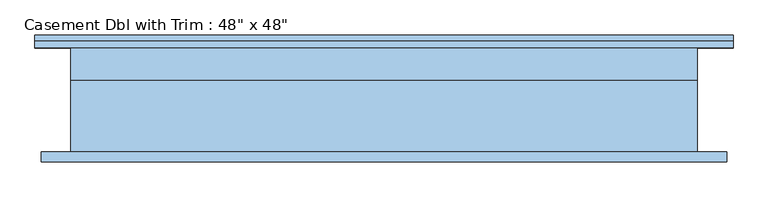
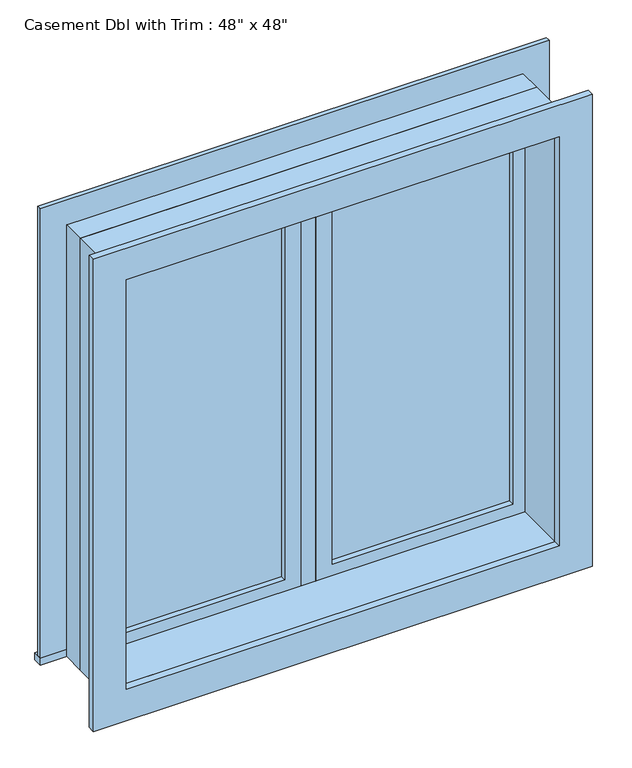
"""IFC4 building model written with IfcOpenShell, lengths in millimetres: window geometry."""

from ifc_helpers import new_model, si_unit, frame, origin, place, context, project, spatial, polyline, outline, extrude, source, transform, mapped, element, save


def window_0862ab64(model_context):
    return source(origin(), model_context, "Body", "SweptSolid", [
        extrude(outline(polyline([(63.5, 85.725), (546.1, 85.725), (546.1, 73.025), (63.5, 73.025), (63.5, 85.725)])), frame((0.0, 0.0, 977.9), z_axis=(0.0, 0.0, 1.0), x_axis=(1.0, 0.0, 0.0)), (0.0, 0.0, 1.0), 1092.2),
        extrude(outline(polyline([(2114.55, 19.05), (933.45, 19.05), (933.45, 590.55), (2114.55, 590.55), (2114.55, 19.05)]), holes=[polyline([(2070.1, 63.5), (2070.1, 546.1), (977.9, 546.1), (977.9, 63.5), (2070.1, 63.5)])]), frame((0.0, 57.15, 0.0), z_axis=(0.0, 1.0, 0.0), x_axis=(0.0, 0.0, 1.0)), (0.0, 0.0, 1.0), 44.45),
        extrude(outline(polyline([(19.05, 57.15), (-19.05, 57.15), (-19.05, 120.65), (19.05, 120.65), (19.05, 57.15)])), frame((0.0, 0.0, 933.45), z_axis=(0.0, 0.0, 1.0), x_axis=(1.0, 0.0, 0.0)), (0.0, 0.0, 1.0), 1181.1),
        extrude(outline(polyline([(-679.45, 146.05), (679.45, 146.05), (679.45, 120.65), (-679.45, 120.65), (-679.45, 146.05)])), frame((0.0, 0.0, 914.4), z_axis=(0.0, 0.0, 1.0), x_axis=(1.0, 0.0, 0.0)), (0.0, 0.0, 1.0), 19.05),
        extrude(outline(polyline([(2114.55, -590.55), (2114.55, 590.55), (933.45, 590.55), (933.45, 679.45), (2203.45, 679.45), (2203.45, -679.45), (933.45, -679.45), (933.45, -590.55), (2114.55, -590.55)])), frame((0.0, 120.65, 0.0), z_axis=(0.0, 1.0, 0.0), x_axis=(0.0, 0.0, 1.0)), (0.0, 0.0, 1.0), 12.7),
        extrude(outline(polyline([(2190.75, 666.75), (2190.75, -666.75), (857.25, -666.75), (857.25, 666.75), (2190.75, 666.75)]), holes=[polyline([(2101.85, 577.85), (946.15, 577.85), (946.15, -577.85), (2101.85, -577.85), (2101.85, 577.85)])]), frame((0.0, -101.6, 0.0), z_axis=(0.0, 1.0, 0.0), x_axis=(0.0, 0.0, 1.0)), (0.0, 0.0, 1.0), 19.05),
        extrude(outline(polyline([(-63.5, 73.025), (-546.1, 73.025), (-546.1, 85.725), (-63.5, 85.725), (-63.5, 73.025)])), frame((0.0, 0.0, 977.9), z_axis=(0.0, 0.0, 1.0), x_axis=(1.0, 0.0, 0.0)), (0.0, 0.0, 1.0), 1092.2),
        extrude(outline(polyline([(2114.55, -590.55), (933.45, -590.55), (933.45, -19.05), (2114.55, -19.05), (2114.55, -590.55)]), holes=[polyline([(2070.1, -546.1), (2070.1, -63.5), (977.9, -63.5), (977.9, -546.1), (2070.1, -546.1)])]), frame((0.0, 57.15, 0.0), z_axis=(0.0, 1.0, 0.0), x_axis=(0.0, 0.0, 1.0)), (0.0, 0.0, 1.0), 44.45),
        extrude(outline(polyline([(2133.6, -609.6), (914.4, -609.6), (914.4, 609.6), (2133.6, 609.6), (2133.6, -609.6)]), holes=[polyline([(2101.85, -577.85), (2101.85, 577.85), (946.15, 577.85), (946.15, -577.85), (2101.85, -577.85)])]), frame((0.0, -82.55, 0.0), z_axis=(0.0, 1.0, 0.0), x_axis=(0.0, 0.0, 1.0)), (0.0, 0.0, 1.0), 139.7),
        extrude(outline(polyline([(2133.6, 609.6), (2133.6, -609.6), (914.4, -609.6), (914.4, 609.6), (2133.6, 609.6)]), holes=[polyline([(2114.55, 590.55), (933.45, 590.55), (933.45, -590.55), (2114.55, -590.55), (2114.55, 590.55)])]), frame((0.0, 57.15, 0.0), z_axis=(0.0, 1.0, 0.0), x_axis=(0.0, 0.0, 1.0)), (0.0, 0.0, 1.0), 63.5),
    ])


if __name__ == "__main__":
    model = new_model("IFC4")
    model_context = context("Model", 3, world=origin())
    ifc_project = project(units=[si_unit("LENGTHUNIT", "METRE", prefix="MILLI")], contexts=[model_context])
    site = spatial("IfcSite", under=ifc_project)
    building = spatial("IfcBuilding", under=site)
    placement = place(None, origin())
    window_shape = window_0862ab64(model_context)
    element("IfcWindow", 1, ObjectType="Casement Dbl with Trim : 48\" x 48\"", at=placement, inside=building, context=model_context, shape_type="MappedRepresentation", body=[
        mapped(window_shape, transform((0.0, 0.0, 0.0), x_axis=(1.0, 0.0, 0.0), y_axis=(0.0, 1.0, 0.0), z_axis=(0.0, 0.0, 1.0))),
    ])
    save(model, "model.ifc")

# Revit data of these elements
# Type "Casement Dbl with Trim : 48\" x 48\""
#   Type Mark = "19"
#   Construction Type Id = "GSP4R"
#   Assembly Code = "B2020100"
#   Analytic Construction = "1/8 in Pilkington single glazing"
#   Visual Light Transmittance = 0.9
#   Solar Heat Gain Coefficient = 0.78
#   Heat Transfer Coefficient (U) = 0.6496 BTU/(h·ft²·°F)
#   Height = 4' - 0"
#   Default Sill Height = 3' - 0"
#   Trim Projection - Ext. = 0' - 0 1/2"
#   Trim Projection - Int. = 0' - 0 3/4"
#   Trim Width - Exterior = 0' - 3 1/2"
#   Trim Width - Interior = 0' - 3 1/2"
#   Width = 4' - 0"
#   Window Inset = 0' - 0 3/4"
#   Define Thermal Properties by = 1
#   Glass Pane Material = Glass
#   Sash Material = Sash
#   Trim Exterior Material = Trim
#   Trim Interior Material = Trim
#   Wall Closure = (empty or 0)
# Element 1 (IfcWindow, "Casement Dbl with Trim : 48\" x 48\"")
#   Materials on its faces: "Sash", "Trim", "Glass"
# Materials
#   "Glass": class "Glass", colour RGB 0 128 192, transparency 0.75, Description = "Soda Lime Glass", Cost = 0
#   "Sash": class "Wood", colour RGB 255 255 255, transparency 0, Cost = 0
#   "Trim": class "Wood", colour RGB 224 178 126, transparency 0
